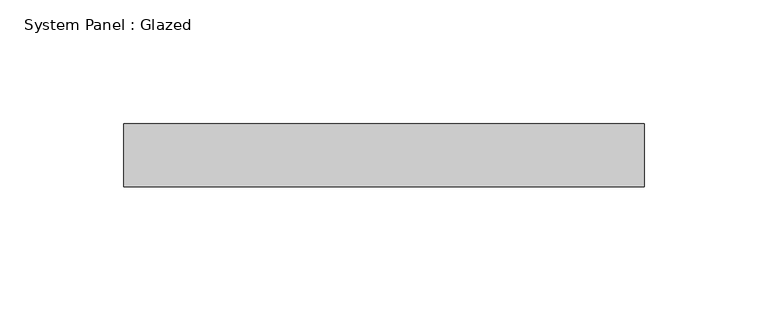
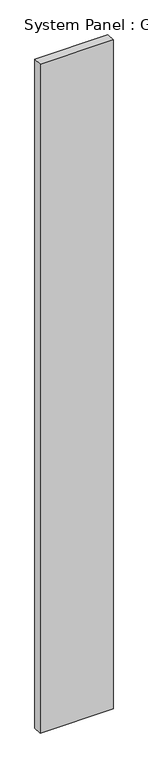
"""IFC4 building model written with IfcOpenShell, lengths in millimetres: plate geometry, System Panel : Glazed."""

from ifc_helpers import new_model, si_unit, origin, origin_with_axes, place, context, project, spatial, polyline, outline, extrude, source, transform, mapped, element, save


def system_panel_glazed_2f540b85(model_context):
    return source(origin(), model_context, "Body", "SweptSolid", [
        extrude(outline(polyline([(104.9570678, 19.05), (-104.9570678, 19.05), (-104.9570678, 44.45), (104.9570678, 44.45), (104.9570678, 19.05)])), origin_with_axes(), (0.0, 0.0, 1.0), 2032.0),
    ])


if __name__ == "__main__":
    model = new_model("IFC4")
    model_context = context("Model", 3, world=origin())
    ifc_project = project(units=[si_unit("LENGTHUNIT", "METRE", prefix="MILLI")], contexts=[model_context])
    site = spatial("IfcSite", under=ifc_project)
    building = spatial("IfcBuilding", under=site)
    placement = place(None, origin())
    system_panel_glazed_shape = system_panel_glazed_2f540b85(model_context)
    element("IfcPlate", 1, ObjectType="System Panel : Glazed", at=placement, inside=building, context=model_context, shape_type="MappedRepresentation", body=[
        mapped(system_panel_glazed_shape, transform((0.0, 0.0, 0.0), x_axis=(1.0, 0.0, 0.0), y_axis=(0.0, 1.0, 0.0), z_axis=(0.0, 0.0, 1.0))),
    ])
    save(model, "model.ifc")

# Revit data of these elements
# Type "System Panel : Glazed"
#   Construction Type Id = "GSP4R"
#   Analytic Construction = "1/8 in Pilkington single glazing"
#   Visual Light Transmittance = 0.9
#   Solar Heat Gain Coefficient = 0.86
#   Heat Transfer Coefficient (U) = 1.18115 BTU/(h·ft²·°F)
# Element 1 (IfcPlate, "System Panel : Glazed")
#   Materials on its faces: "Glass"
# Materials
#   "Glass": class "Glass", colour RGB 0 128 192, transparency 0.75, Description = "Soda Lime Glass", Cost = 0
